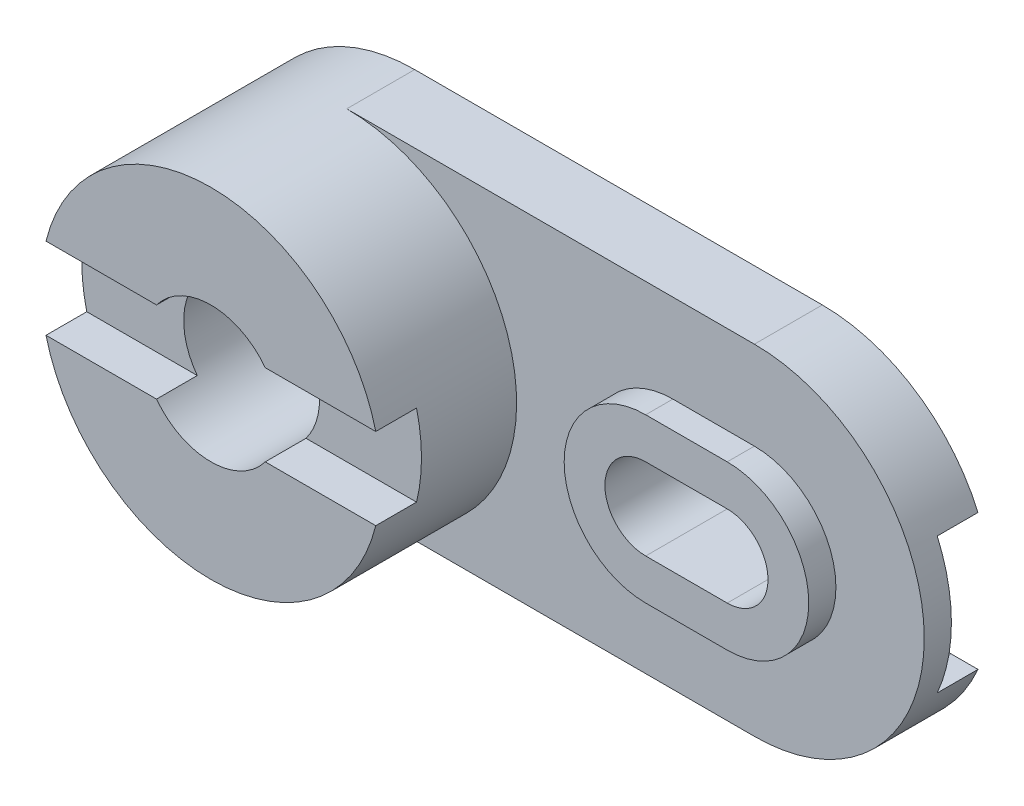
ISO-10303-21;
HEADER;
FILE_DESCRIPTION(('STEP AP214'),'2;1');
FILE_NAME('part.step','',(''),(''),'','','');
FILE_SCHEMA(('AUTOMOTIVE_DESIGN { 1 0 10303 214 1 1 1 1 }'));
ENDSEC;
DATA;
#1=APPLICATION_CONTEXT('core data for automotive mechanical design processes');
#2=APPLICATION_PROTOCOL_DEFINITION('international standard','automotive_design',2000,#1);
#3=PRODUCT_CONTEXT('',#1,'mechanical');
#4=PRODUCT('Part','Part','',(#3));
#5=PRODUCT_RELATED_PRODUCT_CATEGORY('part','',(#4));
#6=PRODUCT_DEFINITION_FORMATION('','',#4);
#7=PRODUCT_DEFINITION_CONTEXT('part definition',#1,'design');
#8=PRODUCT_DEFINITION('design','',#6,#7);
#9=PRODUCT_DEFINITION_SHAPE('','',#8);
#10=(LENGTH_UNIT() NAMED_UNIT(*) SI_UNIT(.MILLI.,.METRE.));
#11=(NAMED_UNIT(*) PLANE_ANGLE_UNIT() SI_UNIT($,.RADIAN.));
#12=(NAMED_UNIT(*) SI_UNIT($,.STERADIAN.) SOLID_ANGLE_UNIT());
#13=UNCERTAINTY_MEASURE_WITH_UNIT(LENGTH_MEASURE(1.E-05),#10,'distance_accuracy_value','');
#14=(GEOMETRIC_REPRESENTATION_CONTEXT(3) GLOBAL_UNCERTAINTY_ASSIGNED_CONTEXT((#13)) GLOBAL_UNIT_ASSIGNED_CONTEXT((#10,
#11,#12)) REPRESENTATION_CONTEXT('',''));
#15=CARTESIAN_POINT('',(0.,0.,0.));
#16=DIRECTION('',(0.,0.,1.));
#17=DIRECTION('',(1.,0.,0.));
#18=AXIS2_PLACEMENT_3D('',#15,#16,#17);
#19=CARTESIAN_POINT('',(60.,0.,10.));
#20=DIRECTION('',(0.,0.,-1.));
#21=DIRECTION('',(-1.,0.,0.));
#22=AXIS2_PLACEMENT_3D('',#19,#20,#21);
#23=CYLINDRICAL_SURFACE('',#22,25.);
#24=DIRECTION('',(0.,0.,1.));
#25=VECTOR('',#24,1.);
#26=CARTESIAN_POINT('',(82.9128784747792,-9.99999999999999,-168.123744974859));
#27=LINE('',#26,#25);
#28=CARTESIAN_POINT('',(82.9128784747792,-9.99999999999999,0.));
#29=VERTEX_POINT('',#28);
#30=CARTESIAN_POINT('',(82.9128784747792,-9.99999999999999,6.));
#31=VERTEX_POINT('',#30);
#32=EDGE_CURVE('E61',#29,#31,#27,.T.);
#33=ORIENTED_EDGE('',*,*,#32,.T.);
#34=CARTESIAN_POINT('',(60.,0.,6.));
#35=DIRECTION('',(0.,0.,1.));
#36=DIRECTION('',(1.,0.,0.));
#37=AXIS2_PLACEMENT_3D('',#34,#35,#36);
#38=CIRCLE('',#37,25.);
#39=CARTESIAN_POINT('',(82.9128784747792,10.,6.));
#40=VERTEX_POINT('',#39);
#41=EDGE_CURVE('E56',#31,#40,#38,.T.);
#42=ORIENTED_EDGE('',*,*,#41,.T.);
#43=DIRECTION('',(0.,0.,1.));
#44=VECTOR('',#43,1.);
#45=CARTESIAN_POINT('',(82.9128784747792,10.,-168.123744974859));
#46=LINE('',#45,#44);
#47=CARTESIAN_POINT('',(82.9128784747792,10.,0.));
#48=VERTEX_POINT('',#47);
#49=EDGE_CURVE('E230',#48,#40,#46,.T.);
#50=ORIENTED_EDGE('',*,*,#49,.F.);
#51=CARTESIAN_POINT('',(60.,0.,0.));
#52=DIRECTION('',(0.,0.,1.));
#53=DIRECTION('',(1.,0.,0.));
#54=AXIS2_PLACEMENT_3D('',#51,#52,#53);
#55=CIRCLE('',#54,25.);
#56=CARTESIAN_POINT('',(60.,25.,0.));
#57=VERTEX_POINT('',#56);
#58=EDGE_CURVE('E213',#48,#57,#55,.T.);
#59=ORIENTED_EDGE('',*,*,#58,.T.);
#60=DIRECTION('',(0.,0.,-1.));
#61=VECTOR('',#60,1.);
#62=CARTESIAN_POINT('',(60.,25.,10.));
#63=LINE('',#62,#61);
#64=CARTESIAN_POINT('',(60.,25.,10.));
#65=VERTEX_POINT('',#64);
#66=EDGE_CURVE('E385',#65,#57,#63,.T.);
#67=ORIENTED_EDGE('',*,*,#66,.F.);
#68=CARTESIAN_POINT('',(60.,0.,10.));
#69=DIRECTION('',(0.,0.,1.));
#70=DIRECTION('',(1.,0.,0.));
#71=AXIS2_PLACEMENT_3D('',#68,#69,#70);
#72=CIRCLE('',#71,25.);
#73=CARTESIAN_POINT('',(60.,-25.,10.));
#74=VERTEX_POINT('',#73);
#75=EDGE_CURVE('E381',#74,#65,#72,.T.);
#76=ORIENTED_EDGE('',*,*,#75,.F.);
#77=DIRECTION('',(0.,0.,-1.));
#78=VECTOR('',#77,1.);
#79=CARTESIAN_POINT('',(60.,-25.,10.));
#80=LINE('',#79,#78);
#81=CARTESIAN_POINT('',(60.,-25.,0.));
#82=VERTEX_POINT('',#81);
#83=EDGE_CURVE('E395',#74,#82,#80,.T.);
#84=ORIENTED_EDGE('',*,*,#83,.T.);
#85=EDGE_CURVE('E223',#82,#29,#55,.T.);
#86=ORIENTED_EDGE('',*,*,#85,.T.);
#87=EDGE_LOOP('',(#33,#42,#50,#59,#67,#76,#84,#86));
#88=FACE_BOUND('',#87,.T.);
#89=ADVANCED_FACE('F44',(#88),#23,.T.);
#90=CARTESIAN_POINT('',(60.,0.,0.));
#91=DIRECTION('',(0.,0.,1.));
#92=DIRECTION('',(1.,0.,0.));
#93=AXIS2_PLACEMENT_3D('',#90,#91,#92);
#94=PLANE('',#93);
#95=CARTESIAN_POINT('',(0.,0.,0.));
#96=DIRECTION('',(0.,0.,1.));
#97=DIRECTION('',(1.,0.,0.));
#98=AXIS2_PLACEMENT_3D('',#95,#96,#97);
#99=CIRCLE('',#98,10.);
#100=CARTESIAN_POINT('',(10.,0.,0.));
#101=VERTEX_POINT('',#100);
#102=EDGE_CURVE('E322',#101,#101,#99,.T.);
#103=ORIENTED_EDGE('',*,*,#102,.T.);
#104=EDGE_LOOP('',(#103));
#105=FACE_BOUND('',#104,.T.);
#106=DIRECTION('',(-1.,0.,0.));
#107=VECTOR('',#106,1.);
#108=CARTESIAN_POINT('',(60.,6.,0.));
#109=LINE('',#108,#107);
#110=CARTESIAN_POINT('',(60.,6.,0.));
#111=VERTEX_POINT('',#110);
#112=CARTESIAN_POINT('',(48.,6.,0.));
#113=VERTEX_POINT('',#112);
#114=EDGE_CURVE('E287',#111,#113,#109,.T.);
#115=ORIENTED_EDGE('',*,*,#114,.T.);
#116=CARTESIAN_POINT('',(48.,0.,0.));
#117=DIRECTION('',(0.,0.,1.));
#118=DIRECTION('',(1.,0.,0.));
#119=AXIS2_PLACEMENT_3D('',#116,#117,#118);
#120=CIRCLE('',#119,6.);
#121=CARTESIAN_POINT('',(48.,-6.,0.));
#122=VERTEX_POINT('',#121);
#123=EDGE_CURVE('E286',#113,#122,#120,.T.);
#124=ORIENTED_EDGE('',*,*,#123,.T.);
#125=DIRECTION('',(1.,0.,0.));
#126=VECTOR('',#125,1.);
#127=CARTESIAN_POINT('',(60.,-6.,0.));
#128=LINE('',#127,#126);
#129=CARTESIAN_POINT('',(60.,-6.,0.));
#130=VERTEX_POINT('',#129);
#131=EDGE_CURVE('E274',#122,#130,#128,.T.);
#132=ORIENTED_EDGE('',*,*,#131,.T.);
#133=CARTESIAN_POINT('',(60.,0.,0.));
#134=DIRECTION('',(0.,0.,1.));
#135=DIRECTION('',(1.,0.,0.));
#136=AXIS2_PLACEMENT_3D('',#133,#134,#135);
#137=CIRCLE('',#136,6.);
#138=EDGE_CURVE('E281',#130,#111,#137,.T.);
#139=ORIENTED_EDGE('',*,*,#138,.T.);
#140=EDGE_LOOP('',(#115,#124,#132,#139));
#141=FACE_BOUND('',#140,.T.);
#142=DIRECTION('',(1.,0.,0.));
#143=VECTOR('',#142,1.);
#144=CARTESIAN_POINT('',(82.9128784747792,-9.99999999999999,0.));
#145=LINE('',#144,#143);
#146=CARTESIAN_POINT('',(79.,-9.99999999999999,0.));
#147=VERTEX_POINT('',#146);
#148=EDGE_CURVE('E258',#147,#29,#145,.T.);
#149=ORIENTED_EDGE('',*,*,#148,.T.);
#150=ORIENTED_EDGE('',*,*,#85,.F.);
#151=DIRECTION('',(1.,0.,0.));
#152=VECTOR('',#151,1.);
#153=CARTESIAN_POINT('',(0.,-25.,0.));
#154=LINE('',#153,#152);
#155=CARTESIAN_POINT('',(0.,-25.,0.));
#156=VERTEX_POINT('',#155);
#157=EDGE_CURVE('E389',#156,#82,#154,.T.);
#158=ORIENTED_EDGE('',*,*,#157,.F.);
#159=CARTESIAN_POINT('',(0.,0.,0.));
#160=DIRECTION('',(0.,0.,1.));
#161=DIRECTION('',(1.,0.,0.));
#162=AXIS2_PLACEMENT_3D('',#159,#160,#161);
#163=CIRCLE('',#162,25.);
#164=CARTESIAN_POINT('',(0.,25.,0.));
#165=VERTEX_POINT('',#164);
#166=EDGE_CURVE('E228',#165,#156,#163,.T.);
#167=ORIENTED_EDGE('',*,*,#166,.F.);
#168=DIRECTION('',(-1.,0.,0.));
#169=VECTOR('',#168,1.);
#170=CARTESIAN_POINT('',(60.,25.,0.));
#171=LINE('',#170,#169);
#172=EDGE_CURVE('E224',#57,#165,#171,.T.);
#173=ORIENTED_EDGE('',*,*,#172,.F.);
#174=ORIENTED_EDGE('',*,*,#58,.F.);
#175=DIRECTION('',(-1.,0.,0.));
#176=VECTOR('',#175,1.);
#177=CARTESIAN_POINT('',(79.,10.,0.));
#178=LINE('',#177,#176);
#179=CARTESIAN_POINT('',(79.,10.,0.));
#180=VERTEX_POINT('',#179);
#181=EDGE_CURVE('E216',#48,#180,#178,.T.);
#182=ORIENTED_EDGE('',*,*,#181,.T.);
#183=DIRECTION('',(-1.,0.,0.));
#184=VECTOR('',#183,1.);
#185=CARTESIAN_POINT('',(79.,10.,0.));
#186=LINE('',#185,#184);
#187=CARTESIAN_POINT('',(69.,10.,0.));
#188=VERTEX_POINT('',#187);
#189=EDGE_CURVE('E237',#180,#188,#186,.T.);
#190=ORIENTED_EDGE('',*,*,#189,.T.);
#191=DIRECTION('',(0.,-1.,0.));
#192=VECTOR('',#191,1.);
#193=CARTESIAN_POINT('',(69.,10.,0.));
#194=LINE('',#193,#192);
#195=CARTESIAN_POINT('',(69.,-9.99999999999999,0.));
#196=VERTEX_POINT('',#195);
#197=EDGE_CURVE('E243',#188,#196,#194,.T.);
#198=ORIENTED_EDGE('',*,*,#197,.T.);
#199=DIRECTION('',(1.,0.,0.));
#200=VECTOR('',#199,1.);
#201=CARTESIAN_POINT('',(69.,-9.99999999999999,0.));
#202=LINE('',#201,#200);
#203=EDGE_CURVE('E435',#196,#147,#202,.T.);
#204=ORIENTED_EDGE('',*,*,#203,.T.);
#205=EDGE_LOOP('',(#149,#150,#158,#167,#173,#174,#182,#190,#198,#204));
#206=FACE_BOUND('',#205,.T.);
#207=ADVANCED_FACE('F218',(#105,#141,#206),#94,.F.);
#208=CARTESIAN_POINT('',(60.,0.,10.));
#209=DIRECTION('',(0.,0.,1.));
#210=DIRECTION('',(1.,0.,0.));
#211=AXIS2_PLACEMENT_3D('',#208,#209,#210);
#212=PLANE('',#211);
#213=CARTESIAN_POINT('',(0.,0.,10.));
#214=DIRECTION('',(0.,0.,1.));
#215=DIRECTION('',(1.,0.,0.));
#216=AXIS2_PLACEMENT_3D('',#213,#214,#215);
#217=CIRCLE('',#216,25.);
#218=CARTESIAN_POINT('',(0.,-25.,10.));
#219=VERTEX_POINT('',#218);
#220=CARTESIAN_POINT('',(0.,25.,10.));
#221=VERTEX_POINT('',#220);
#222=EDGE_CURVE('E378',#219,#221,#217,.T.);
#223=ORIENTED_EDGE('',*,*,#222,.F.);
#224=DIRECTION('',(1.,0.,0.));
#225=VECTOR('',#224,1.);
#226=CARTESIAN_POINT('',(0.,-25.,10.));
#227=LINE('',#226,#225);
#228=EDGE_CURVE('E393',#219,#74,#227,.T.);
#229=ORIENTED_EDGE('',*,*,#228,.T.);
#230=ORIENTED_EDGE('',*,*,#75,.T.);
#231=DIRECTION('',(-1.,0.,0.));
#232=VECTOR('',#231,1.);
#233=CARTESIAN_POINT('',(60.,25.,10.));
#234=LINE('',#233,#232);
#235=EDGE_CURVE('E390',#65,#221,#234,.T.);
#236=ORIENTED_EDGE('',*,*,#235,.T.);
#237=EDGE_LOOP('',(#223,#229,#230,#236));
#238=FACE_BOUND('',#237,.T.);
#239=DIRECTION('',(1.,0.,0.));
#240=VECTOR('',#239,1.);
#241=CARTESIAN_POINT('',(48.,-12.,10.));
#242=LINE('',#241,#240);
#243=CARTESIAN_POINT('',(48.,-12.,10.));
#244=VERTEX_POINT('',#243);
#245=CARTESIAN_POINT('',(60.,-12.,10.));
#246=VERTEX_POINT('',#245);
#247=EDGE_CURVE('E306',#244,#246,#242,.T.);
#248=ORIENTED_EDGE('',*,*,#247,.F.);
#249=CARTESIAN_POINT('',(48.,0.,10.));
#250=DIRECTION('',(0.,0.,1.));
#251=DIRECTION('',(1.,0.,0.));
#252=AXIS2_PLACEMENT_3D('',#249,#250,#251);
#253=CIRCLE('',#252,12.);
#254=CARTESIAN_POINT('',(48.,12.,10.));
#255=VERTEX_POINT('',#254);
#256=EDGE_CURVE('E292',#255,#244,#253,.T.);
#257=ORIENTED_EDGE('',*,*,#256,.F.);
#258=DIRECTION('',(-1.,0.,0.));
#259=VECTOR('',#258,1.);
#260=CARTESIAN_POINT('',(48.,12.,10.));
#261=LINE('',#260,#259);
#262=CARTESIAN_POINT('',(60.,12.,10.));
#263=VERTEX_POINT('',#262);
#264=EDGE_CURVE('E300',#263,#255,#261,.T.);
#265=ORIENTED_EDGE('',*,*,#264,.F.);
#266=CARTESIAN_POINT('',(60.,0.,10.));
#267=DIRECTION('',(0.,0.,1.));
#268=DIRECTION('',(1.,0.,0.));
#269=AXIS2_PLACEMENT_3D('',#266,#267,#268);
#270=CIRCLE('',#269,12.);
#271=EDGE_CURVE('E308',#246,#263,#270,.T.);
#272=ORIENTED_EDGE('',*,*,#271,.F.);
#273=EDGE_LOOP('',(#248,#257,#265,#272));
#274=FACE_BOUND('',#273,.T.);
#275=ADVANCED_FACE('F409',(#238,#274),#212,.T.);
#276=CARTESIAN_POINT('',(0.,0.,24.));
#277=DIRECTION('',(0.,0.,1.));
#278=DIRECTION('',(1.,0.,0.));
#279=AXIS2_PLACEMENT_3D('',#276,#277,#278);
#280=PLANE('',#279);
#281=CARTESIAN_POINT('',(0.,0.,24.));
#282=DIRECTION('',(0.,0.,1.));
#283=DIRECTION('',(1.,0.,0.));
#284=AXIS2_PLACEMENT_3D('',#281,#282,#283);
#285=CIRCLE('',#284,10.);
#286=CARTESIAN_POINT('',(-8.,6.,24.));
#287=VERTEX_POINT('',#286);
#288=CARTESIAN_POINT('',(-8.,-6.,24.));
#289=VERTEX_POINT('',#288);
#290=EDGE_CURVE('E11',#287,#289,#285,.T.);
#291=ORIENTED_EDGE('',*,*,#290,.F.);
#292=DIRECTION('',(1.,0.,0.));
#293=VECTOR('',#292,1.);
#294=CARTESIAN_POINT('',(0.,6.,24.));
#295=LINE('',#294,#293);
#296=CARTESIAN_POINT('',(-24.2693221990232,6.,24.));
#297=VERTEX_POINT('',#296);
#298=EDGE_CURVE('E330',#297,#287,#295,.T.);
#299=ORIENTED_EDGE('',*,*,#298,.F.);
#300=CARTESIAN_POINT('',(0.,0.,24.));
#301=DIRECTION('',(0.,0.,1.));
#302=DIRECTION('',(1.,0.,0.));
#303=AXIS2_PLACEMENT_3D('',#300,#301,#302);
#304=CIRCLE('',#303,25.);
#305=CARTESIAN_POINT('',(-24.2693221990232,-6.,24.));
#306=VERTEX_POINT('',#305);
#307=EDGE_CURVE('E332',#297,#306,#304,.T.);
#308=ORIENTED_EDGE('',*,*,#307,.T.);
#309=DIRECTION('',(-1.,0.,0.));
#310=VECTOR('',#309,1.);
#311=CARTESIAN_POINT('',(0.,-6.,24.));
#312=LINE('',#311,#310);
#313=EDGE_CURVE('E331',#289,#306,#312,.T.);
#314=ORIENTED_EDGE('',*,*,#313,.F.);
#315=EDGE_LOOP('',(#291,#299,#308,#314));
#316=FACE_BOUND('',#315,.T.);
#317=ADVANCED_FACE('F465',(#316),#280,.T.);
#318=CARTESIAN_POINT('',(0.,0.,0.));
#319=DIRECTION('',(0.,0.,1.));
#320=DIRECTION('',(1.,0.,0.));
#321=AXIS2_PLACEMENT_3D('',#318,#319,#320);
#322=CYLINDRICAL_SURFACE('',#321,25.);
#323=DIRECTION('',(0.,0.,-1.));
#324=VECTOR('',#323,1.);
#325=CARTESIAN_POINT('',(0.,25.,10.));
#326=LINE('',#325,#324);
#327=EDGE_CURVE('E402',#221,#165,#326,.T.);
#328=ORIENTED_EDGE('',*,*,#327,.T.);
#329=ORIENTED_EDGE('',*,*,#166,.T.);
#330=DIRECTION('',(0.,0.,-1.));
#331=VECTOR('',#330,1.);
#332=CARTESIAN_POINT('',(0.,-25.,10.));
#333=LINE('',#332,#331);
#334=EDGE_CURVE('E400',#219,#156,#333,.T.);
#335=ORIENTED_EDGE('',*,*,#334,.F.);
#336=ORIENTED_EDGE('',*,*,#222,.T.);
#337=EDGE_LOOP('',(#328,#329,#335,#336));
#338=FACE_BOUND('',#337,.T.);
#339=CARTESIAN_POINT('',(0.,0.,30.));
#340=DIRECTION('',(0.,0.,1.));
#341=DIRECTION('',(1.,0.,0.));
#342=AXIS2_PLACEMENT_3D('',#339,#340,#341);
#343=CIRCLE('',#342,25.);
#344=CARTESIAN_POINT('',(-24.2693221990232,-6.,30.));
#345=VERTEX_POINT('',#344);
#346=CARTESIAN_POINT('',(24.2693221990232,-6.,30.));
#347=VERTEX_POINT('',#346);
#348=EDGE_CURVE('E356',#345,#347,#343,.T.);
#349=ORIENTED_EDGE('',*,*,#348,.F.);
#350=DIRECTION('',(0.,0.,1.));
#351=VECTOR('',#350,1.);
#352=CARTESIAN_POINT('',(-24.2693221990232,-6.,24.));
#353=LINE('',#352,#351);
#354=EDGE_CURVE('E366',#306,#345,#353,.T.);
#355=ORIENTED_EDGE('',*,*,#354,.F.);
#356=ORIENTED_EDGE('',*,*,#307,.F.);
#357=DIRECTION('',(0.,0.,1.));
#358=VECTOR('',#357,1.);
#359=CARTESIAN_POINT('',(-24.2693221990232,6.,24.));
#360=LINE('',#359,#358);
#361=CARTESIAN_POINT('',(-24.2693221990232,6.,30.));
#362=VERTEX_POINT('',#361);
#363=EDGE_CURVE('E368',#297,#362,#360,.T.);
#364=ORIENTED_EDGE('',*,*,#363,.T.);
#365=CARTESIAN_POINT('',(24.2693221990232,6.,30.));
#366=VERTEX_POINT('',#365);
#367=EDGE_CURVE('E376',#366,#362,#343,.T.);
#368=ORIENTED_EDGE('',*,*,#367,.F.);
#369=DIRECTION('',(0.,0.,1.));
#370=VECTOR('',#369,1.);
#371=CARTESIAN_POINT('',(24.2693221990232,6.,24.));
#372=LINE('',#371,#370);
#373=CARTESIAN_POINT('',(24.2693221990232,6.,24.));
#374=VERTEX_POINT('',#373);
#375=EDGE_CURVE('E358',#374,#366,#372,.T.);
#376=ORIENTED_EDGE('',*,*,#375,.F.);
#377=CARTESIAN_POINT('',(24.2693221990232,-6.,24.));
#378=VERTEX_POINT('',#377);
#379=EDGE_CURVE('E333',#378,#374,#304,.T.);
#380=ORIENTED_EDGE('',*,*,#379,.F.);
#381=DIRECTION('',(0.,0.,1.));
#382=VECTOR('',#381,1.);
#383=CARTESIAN_POINT('',(24.2693221990232,-6.,24.));
#384=LINE('',#383,#382);
#385=EDGE_CURVE('E360',#378,#347,#384,.T.);
#386=ORIENTED_EDGE('',*,*,#385,.T.);
#387=EDGE_LOOP('',(#349,#355,#356,#364,#368,#376,#380,#386));
#388=FACE_BOUND('',#387,.T.);
#389=ADVANCED_FACE('F484',(#338,#388),#322,.T.);
#390=CARTESIAN_POINT('',(0.,0.,30.));
#391=DIRECTION('',(0.,0.,1.));
#392=DIRECTION('',(1.,0.,0.));
#393=AXIS2_PLACEMENT_3D('',#390,#391,#392);
#394=PLANE('',#393);
#395=ORIENTED_EDGE('',*,*,#348,.T.);
#396=DIRECTION('',(-1.,0.,0.));
#397=VECTOR('',#396,1.);
#398=CARTESIAN_POINT('',(0.,-6.,30.));
#399=LINE('',#398,#397);
#400=CARTESIAN_POINT('',(8.,-6.,30.));
#401=VERTEX_POINT('',#400);
#402=EDGE_CURVE('E326',#347,#401,#399,.T.);
#403=ORIENTED_EDGE('',*,*,#402,.T.);
#404=CARTESIAN_POINT('',(0.,0.,30.));
#405=DIRECTION('',(0.,0.,1.));
#406=DIRECTION('',(1.,0.,0.));
#407=AXIS2_PLACEMENT_3D('',#404,#405,#406);
#408=CIRCLE('',#407,10.);
#409=CARTESIAN_POINT('',(-8.,-6.,30.));
#410=VERTEX_POINT('',#409);
#411=EDGE_CURVE('E352',#410,#401,#408,.T.);
#412=ORIENTED_EDGE('',*,*,#411,.F.);
#413=DIRECTION('',(-1.,0.,0.));
#414=VECTOR('',#413,1.);
#415=CARTESIAN_POINT('',(0.,-6.,30.));
#416=LINE('',#415,#414);
#417=EDGE_CURVE('E346',#410,#345,#416,.T.);
#418=ORIENTED_EDGE('',*,*,#417,.T.);
#419=EDGE_LOOP('',(#395,#403,#412,#418));
#420=FACE_BOUND('',#419,.T.);
#421=ADVANCED_FACE('F473',(#420),#394,.T.);
#422=CARTESIAN_POINT('',(0.,0.,30.));
#423=DIRECTION('',(0.,0.,1.));
#424=DIRECTION('',(1.,0.,0.));
#425=AXIS2_PLACEMENT_3D('',#422,#423,#424);
#426=CIRCLE('',#425,10.);
#427=CARTESIAN_POINT('',(8.,6.,30.));
#428=VERTEX_POINT('',#427);
#429=CARTESIAN_POINT('',(-8.,6.,30.));
#430=VERTEX_POINT('',#429);
#431=EDGE_CURVE('E345',#428,#430,#426,.T.);
#432=ORIENTED_EDGE('',*,*,#431,.F.);
#433=DIRECTION('',(1.,0.,0.));
#434=VECTOR('',#433,1.);
#435=CARTESIAN_POINT('',(0.,6.,30.));
#436=LINE('',#435,#434);
#437=EDGE_CURVE('E321',#428,#366,#436,.T.);
#438=ORIENTED_EDGE('',*,*,#437,.T.);
#439=ORIENTED_EDGE('',*,*,#367,.T.);
#440=DIRECTION('',(1.,0.,0.));
#441=VECTOR('',#440,1.);
#442=CARTESIAN_POINT('',(0.,6.,30.));
#443=LINE('',#442,#441);
#444=EDGE_CURVE('E343',#362,#430,#443,.T.);
#445=ORIENTED_EDGE('',*,*,#444,.T.);
#446=EDGE_LOOP('',(#432,#438,#439,#445));
#447=FACE_BOUND('',#446,.T.);
#448=ADVANCED_FACE('F472',(#447),#394,.T.);
#449=CARTESIAN_POINT('',(60.,25.,10.));
#450=DIRECTION('',(0.,-1.,0.));
#451=DIRECTION('',(0.,0.,-1.));
#452=AXIS2_PLACEMENT_3D('',#449,#450,#451);
#453=PLANE('',#452);
#454=ORIENTED_EDGE('',*,*,#172,.T.);
#455=ORIENTED_EDGE('',*,*,#327,.F.);
#456=ORIENTED_EDGE('',*,*,#235,.F.);
#457=ORIENTED_EDGE('',*,*,#66,.T.);
#458=EDGE_LOOP('',(#454,#455,#456,#457));
#459=FACE_BOUND('',#458,.T.);
#460=ADVANCED_FACE('F401',(#459),#453,.F.);
#461=CARTESIAN_POINT('',(0.,-25.,10.));
#462=DIRECTION('',(0.,1.,0.));
#463=DIRECTION('',(0.,0.,1.));
#464=AXIS2_PLACEMENT_3D('',#461,#462,#463);
#465=PLANE('',#464);
#466=ORIENTED_EDGE('',*,*,#157,.T.);
#467=ORIENTED_EDGE('',*,*,#83,.F.);
#468=ORIENTED_EDGE('',*,*,#228,.F.);
#469=ORIENTED_EDGE('',*,*,#334,.T.);
#470=EDGE_LOOP('',(#466,#467,#468,#469));
#471=FACE_BOUND('',#470,.T.);
#472=ADVANCED_FACE('F411',(#471),#465,.F.);
#473=CARTESIAN_POINT('',(0.,6.,24.));
#474=DIRECTION('',(0.,-1.,0.));
#475=DIRECTION('',(1.,0.,0.));
#476=AXIS2_PLACEMENT_3D('',#473,#474,#475);
#477=PLANE('',#476);
#478=ORIENTED_EDGE('',*,*,#437,.F.);
#479=DIRECTION('',(0.,0.,1.));
#480=VECTOR('',#479,1.);
#481=CARTESIAN_POINT('',(8.,6.,24.));
#482=LINE('',#481,#480);
#483=CARTESIAN_POINT('',(8.,6.,24.));
#484=VERTEX_POINT('',#483);
#485=EDGE_CURVE('E373',#484,#428,#482,.T.);
#486=ORIENTED_EDGE('',*,*,#485,.F.);
#487=DIRECTION('',(1.,0.,0.));
#488=VECTOR('',#487,1.);
#489=CARTESIAN_POINT('',(0.,6.,24.));
#490=LINE('',#489,#488);
#491=EDGE_CURVE('E323',#484,#374,#490,.T.);
#492=ORIENTED_EDGE('',*,*,#491,.T.);
#493=ORIENTED_EDGE('',*,*,#375,.T.);
#494=EDGE_LOOP('',(#478,#486,#492,#493));
#495=FACE_BOUND('',#494,.T.);
#496=ADVANCED_FACE('F469',(#495),#477,.T.);
#497=CARTESIAN_POINT('',(0.,-6.,24.));
#498=DIRECTION('',(0.,1.,0.));
#499=DIRECTION('',(-1.,0.,0.));
#500=AXIS2_PLACEMENT_3D('',#497,#498,#499);
#501=PLANE('',#500);
#502=ORIENTED_EDGE('',*,*,#402,.F.);
#503=ORIENTED_EDGE('',*,*,#385,.F.);
#504=DIRECTION('',(-1.,0.,0.));
#505=VECTOR('',#504,1.);
#506=CARTESIAN_POINT('',(0.,-6.,24.));
#507=LINE('',#506,#505);
#508=CARTESIAN_POINT('',(8.,-6.,24.));
#509=VERTEX_POINT('',#508);
#510=EDGE_CURVE('E340',#378,#509,#507,.T.);
#511=ORIENTED_EDGE('',*,*,#510,.T.);
#512=DIRECTION('',(0.,0.,1.));
#513=VECTOR('',#512,1.);
#514=CARTESIAN_POINT('',(8.,-6.,24.));
#515=LINE('',#514,#513);
#516=EDGE_CURVE('E365',#509,#401,#515,.T.);
#517=ORIENTED_EDGE('',*,*,#516,.T.);
#518=EDGE_LOOP('',(#502,#503,#511,#517));
#519=FACE_BOUND('',#518,.T.);
#520=ADVANCED_FACE('F521',(#519),#501,.T.);
#521=CARTESIAN_POINT('',(0.,0.,24.));
#522=DIRECTION('',(0.,0.,1.));
#523=DIRECTION('',(1.,0.,0.));
#524=AXIS2_PLACEMENT_3D('',#521,#522,#523);
#525=CYLINDRICAL_SURFACE('',#524,10.);
#526=ORIENTED_EDGE('',*,*,#411,.T.);
#527=ORIENTED_EDGE('',*,*,#516,.F.);
#528=EDGE_CURVE('E48',#509,#484,#285,.T.);
#529=ORIENTED_EDGE('',*,*,#528,.T.);
#530=ORIENTED_EDGE('',*,*,#485,.T.);
#531=ORIENTED_EDGE('',*,*,#431,.T.);
#532=DIRECTION('',(0.,0.,1.));
#533=VECTOR('',#532,1.);
#534=CARTESIAN_POINT('',(-8.,6.,24.));
#535=LINE('',#534,#533);
#536=EDGE_CURVE('E371',#287,#430,#535,.T.);
#537=ORIENTED_EDGE('',*,*,#536,.F.);
#538=ORIENTED_EDGE('',*,*,#290,.T.);
#539=DIRECTION('',(0.,0.,1.));
#540=VECTOR('',#539,1.);
#541=CARTESIAN_POINT('',(-8.,-6.,24.));
#542=LINE('',#541,#540);
#543=EDGE_CURVE('E364',#289,#410,#542,.T.);
#544=ORIENTED_EDGE('',*,*,#543,.T.);
#545=EDGE_LOOP('',(#526,#527,#529,#530,#531,#537,#538,#544));
#546=FACE_BOUND('',#545,.T.);
#547=ORIENTED_EDGE('',*,*,#102,.F.);
#548=EDGE_LOOP('',(#547));
#549=FACE_BOUND('',#548,.T.);
#550=ADVANCED_FACE('F513',(#546,#549),#525,.F.);
#551=CARTESIAN_POINT('',(0.,-6.,24.));
#552=DIRECTION('',(0.,1.,0.));
#553=DIRECTION('',(-1.,0.,0.));
#554=AXIS2_PLACEMENT_3D('',#551,#552,#553);
#555=PLANE('',#554);
#556=ORIENTED_EDGE('',*,*,#417,.F.);
#557=ORIENTED_EDGE('',*,*,#543,.F.);
#558=ORIENTED_EDGE('',*,*,#313,.T.);
#559=ORIENTED_EDGE('',*,*,#354,.T.);
#560=EDGE_LOOP('',(#556,#557,#558,#559));
#561=FACE_BOUND('',#560,.T.);
#562=ADVANCED_FACE('F504',(#561),#555,.T.);
#563=CARTESIAN_POINT('',(0.,6.,24.));
#564=DIRECTION('',(0.,-1.,0.));
#565=DIRECTION('',(1.,0.,0.));
#566=AXIS2_PLACEMENT_3D('',#563,#564,#565);
#567=PLANE('',#566);
#568=ORIENTED_EDGE('',*,*,#444,.F.);
#569=ORIENTED_EDGE('',*,*,#363,.F.);
#570=ORIENTED_EDGE('',*,*,#298,.T.);
#571=ORIENTED_EDGE('',*,*,#536,.T.);
#572=EDGE_LOOP('',(#568,#569,#570,#571));
#573=FACE_BOUND('',#572,.T.);
#574=ADVANCED_FACE('F522',(#573),#567,.T.);
#575=ORIENTED_EDGE('',*,*,#528,.F.);
#576=ORIENTED_EDGE('',*,*,#510,.F.);
#577=ORIENTED_EDGE('',*,*,#379,.T.);
#578=ORIENTED_EDGE('',*,*,#491,.F.);
#579=EDGE_LOOP('',(#575,#576,#577,#578));
#580=FACE_BOUND('',#579,.T.);
#581=ADVANCED_FACE('F494',(#580),#280,.T.);
#582=CARTESIAN_POINT('',(48.,0.,14.));
#583=DIRECTION('',(0.,0.,-1.));
#584=DIRECTION('',(-1.,0.,0.));
#585=AXIS2_PLACEMENT_3D('',#582,#583,#584);
#586=CYLINDRICAL_SURFACE('',#585,12.);
#587=ORIENTED_EDGE('',*,*,#256,.T.);
#588=DIRECTION('',(0.,0.,-1.));
#589=VECTOR('',#588,1.);
#590=CARTESIAN_POINT('',(48.,-12.,14.));
#591=LINE('',#590,#589);
#592=CARTESIAN_POINT('',(48.,-12.,14.));
#593=VERTEX_POINT('',#592);
#594=EDGE_CURVE('E316',#593,#244,#591,.T.);
#595=ORIENTED_EDGE('',*,*,#594,.F.);
#596=CARTESIAN_POINT('',(48.,0.,14.));
#597=DIRECTION('',(0.,0.,1.));
#598=DIRECTION('',(1.,0.,0.));
#599=AXIS2_PLACEMENT_3D('',#596,#597,#598);
#600=CIRCLE('',#599,12.);
#601=CARTESIAN_POINT('',(48.,12.,14.));
#602=VERTEX_POINT('',#601);
#603=EDGE_CURVE('E291',#602,#593,#600,.T.);
#604=ORIENTED_EDGE('',*,*,#603,.F.);
#605=DIRECTION('',(0.,0.,-1.));
#606=VECTOR('',#605,1.);
#607=CARTESIAN_POINT('',(48.,12.,14.));
#608=LINE('',#607,#606);
#609=EDGE_CURVE('E303',#602,#255,#608,.T.);
#610=ORIENTED_EDGE('',*,*,#609,.T.);
#611=EDGE_LOOP('',(#587,#595,#604,#610));
#612=FACE_BOUND('',#611,.T.);
#613=ADVANCED_FACE('F528',(#612),#586,.T.);
#614=CARTESIAN_POINT('',(48.,-12.,14.));
#615=DIRECTION('',(0.,1.,0.));
#616=DIRECTION('',(0.,0.,1.));
#617=AXIS2_PLACEMENT_3D('',#614,#615,#616);
#618=PLANE('',#617);
#619=ORIENTED_EDGE('',*,*,#247,.T.);
#620=DIRECTION('',(0.,0.,-1.));
#621=VECTOR('',#620,1.);
#622=CARTESIAN_POINT('',(60.,-12.,14.));
#623=LINE('',#622,#621);
#624=CARTESIAN_POINT('',(60.,-12.,14.));
#625=VERTEX_POINT('',#624);
#626=EDGE_CURVE('E317',#625,#246,#623,.T.);
#627=ORIENTED_EDGE('',*,*,#626,.F.);
#628=DIRECTION('',(1.,0.,0.));
#629=VECTOR('',#628,1.);
#630=CARTESIAN_POINT('',(48.,-12.,14.));
#631=LINE('',#630,#629);
#632=EDGE_CURVE('E298',#593,#625,#631,.T.);
#633=ORIENTED_EDGE('',*,*,#632,.F.);
#634=ORIENTED_EDGE('',*,*,#594,.T.);
#635=EDGE_LOOP('',(#619,#627,#633,#634));
#636=FACE_BOUND('',#635,.T.);
#637=ADVANCED_FACE('F536',(#636),#618,.F.);
#638=CARTESIAN_POINT('',(60.,0.,14.));
#639=DIRECTION('',(0.,0.,-1.));
#640=DIRECTION('',(-1.,0.,0.));
#641=AXIS2_PLACEMENT_3D('',#638,#639,#640);
#642=CYLINDRICAL_SURFACE('',#641,12.);
#643=ORIENTED_EDGE('',*,*,#271,.T.);
#644=DIRECTION('',(0.,0.,-1.));
#645=VECTOR('',#644,1.);
#646=CARTESIAN_POINT('',(60.,12.,14.));
#647=LINE('',#646,#645);
#648=CARTESIAN_POINT('',(60.,12.,14.));
#649=VERTEX_POINT('',#648);
#650=EDGE_CURVE('E313',#649,#263,#647,.T.);
#651=ORIENTED_EDGE('',*,*,#650,.F.);
#652=CARTESIAN_POINT('',(60.,0.,14.));
#653=DIRECTION('',(0.,0.,1.));
#654=DIRECTION('',(1.,0.,0.));
#655=AXIS2_PLACEMENT_3D('',#652,#653,#654);
#656=CIRCLE('',#655,12.);
#657=EDGE_CURVE('E299',#625,#649,#656,.T.);
#658=ORIENTED_EDGE('',*,*,#657,.F.);
#659=ORIENTED_EDGE('',*,*,#626,.T.);
#660=EDGE_LOOP('',(#643,#651,#658,#659));
#661=FACE_BOUND('',#660,.T.);
#662=ADVANCED_FACE('F541',(#661),#642,.T.);
#663=CARTESIAN_POINT('',(48.,12.,14.));
#664=DIRECTION('',(0.,-1.,0.));
#665=DIRECTION('',(0.,0.,-1.));
#666=AXIS2_PLACEMENT_3D('',#663,#664,#665);
#667=PLANE('',#666);
#668=ORIENTED_EDGE('',*,*,#264,.T.);
#669=ORIENTED_EDGE('',*,*,#609,.F.);
#670=DIRECTION('',(-1.,0.,0.));
#671=VECTOR('',#670,1.);
#672=CARTESIAN_POINT('',(48.,12.,14.));
#673=LINE('',#672,#671);
#674=EDGE_CURVE('E301',#649,#602,#673,.T.);
#675=ORIENTED_EDGE('',*,*,#674,.F.);
#676=ORIENTED_EDGE('',*,*,#650,.T.);
#677=EDGE_LOOP('',(#668,#669,#675,#676));
#678=FACE_BOUND('',#677,.T.);
#679=ADVANCED_FACE('F549',(#678),#667,.F.);
#680=CARTESIAN_POINT('',(48.,0.,14.));
#681=DIRECTION('',(0.,0.,1.));
#682=DIRECTION('',(1.,0.,0.));
#683=AXIS2_PLACEMENT_3D('',#680,#681,#682);
#684=PLANE('',#683);
#685=CARTESIAN_POINT('',(48.,0.,14.));
#686=DIRECTION('',(0.,0.,1.));
#687=DIRECTION('',(1.,0.,0.));
#688=AXIS2_PLACEMENT_3D('',#685,#686,#687);
#689=CIRCLE('',#688,6.);
#690=CARTESIAN_POINT('',(48.,6.,14.));
#691=VERTEX_POINT('',#690);
#692=CARTESIAN_POINT('',(48.,-6.,14.));
#693=VERTEX_POINT('',#692);
#694=EDGE_CURVE('E259',#691,#693,#689,.T.);
#695=ORIENTED_EDGE('',*,*,#694,.F.);
#696=DIRECTION('',(-1.,0.,0.));
#697=VECTOR('',#696,1.);
#698=CARTESIAN_POINT('',(48.,6.,14.));
#699=LINE('',#698,#697);
#700=CARTESIAN_POINT('',(60.,6.,14.));
#701=VERTEX_POINT('',#700);
#702=EDGE_CURVE('E270',#701,#691,#699,.T.);
#703=ORIENTED_EDGE('',*,*,#702,.F.);
#704=CARTESIAN_POINT('',(60.,0.,14.));
#705=DIRECTION('',(0.,0.,1.));
#706=DIRECTION('',(1.,0.,0.));
#707=AXIS2_PLACEMENT_3D('',#704,#705,#706);
#708=CIRCLE('',#707,6.);
#709=CARTESIAN_POINT('',(60.,-6.,14.));
#710=VERTEX_POINT('',#709);
#711=EDGE_CURVE('E264',#710,#701,#708,.T.);
#712=ORIENTED_EDGE('',*,*,#711,.F.);
#713=DIRECTION('',(1.,0.,0.));
#714=VECTOR('',#713,1.);
#715=CARTESIAN_POINT('',(60.,-6.,14.));
#716=LINE('',#715,#714);
#717=EDGE_CURVE('E265',#693,#710,#716,.T.);
#718=ORIENTED_EDGE('',*,*,#717,.F.);
#719=EDGE_LOOP('',(#695,#703,#712,#718));
#720=FACE_BOUND('',#719,.T.);
#721=ORIENTED_EDGE('',*,*,#603,.T.);
#722=ORIENTED_EDGE('',*,*,#632,.T.);
#723=ORIENTED_EDGE('',*,*,#657,.T.);
#724=ORIENTED_EDGE('',*,*,#674,.T.);
#725=EDGE_LOOP('',(#721,#722,#723,#724));
#726=FACE_BOUND('',#725,.T.);
#727=ADVANCED_FACE('F553',(#720,#726),#684,.T.);
#728=CARTESIAN_POINT('',(48.,0.,-6.));
#729=DIRECTION('',(0.,0.,1.));
#730=DIRECTION('',(1.,0.,0.));
#731=AXIS2_PLACEMENT_3D('',#728,#729,#730);
#732=CYLINDRICAL_SURFACE('',#731,6.);
#733=DIRECTION('',(0.,0.,1.));
#734=VECTOR('',#733,1.);
#735=CARTESIAN_POINT('',(48.,6.,-6.));
#736=LINE('',#735,#734);
#737=EDGE_CURVE('E275',#113,#691,#736,.T.);
#738=ORIENTED_EDGE('',*,*,#737,.T.);
#739=ORIENTED_EDGE('',*,*,#694,.T.);
#740=DIRECTION('',(0.,0.,1.));
#741=VECTOR('',#740,1.);
#742=CARTESIAN_POINT('',(48.,-6.,-6.));
#743=LINE('',#742,#741);
#744=EDGE_CURVE('E272',#122,#693,#743,.T.);
#745=ORIENTED_EDGE('',*,*,#744,.F.);
#746=ORIENTED_EDGE('',*,*,#123,.F.);
#747=EDGE_LOOP('',(#738,#739,#745,#746));
#748=FACE_BOUND('',#747,.T.);
#749=ADVANCED_FACE('F554',(#748),#732,.F.);
#750=CARTESIAN_POINT('',(48.,6.,-6.));
#751=DIRECTION('',(0.,1.,0.));
#752=DIRECTION('',(0.,0.,1.));
#753=AXIS2_PLACEMENT_3D('',#750,#751,#752);
#754=PLANE('',#753);
#755=DIRECTION('',(0.,0.,1.));
#756=VECTOR('',#755,1.);
#757=CARTESIAN_POINT('',(60.,6.,-6.));
#758=LINE('',#757,#756);
#759=EDGE_CURVE('E273',#111,#701,#758,.T.);
#760=ORIENTED_EDGE('',*,*,#759,.T.);
#761=ORIENTED_EDGE('',*,*,#702,.T.);
#762=ORIENTED_EDGE('',*,*,#737,.F.);
#763=ORIENTED_EDGE('',*,*,#114,.F.);
#764=EDGE_LOOP('',(#760,#761,#762,#763));
#765=FACE_BOUND('',#764,.T.);
#766=ADVANCED_FACE('F559',(#765),#754,.F.);
#767=CARTESIAN_POINT('',(60.,0.,-6.));
#768=DIRECTION('',(0.,0.,1.));
#769=DIRECTION('',(1.,0.,0.));
#770=AXIS2_PLACEMENT_3D('',#767,#768,#769);
#771=CYLINDRICAL_SURFACE('',#770,6.);
#772=DIRECTION('',(0.,0.,1.));
#773=VECTOR('',#772,1.);
#774=CARTESIAN_POINT('',(60.,-6.,-6.));
#775=LINE('',#774,#773);
#776=EDGE_CURVE('E280',#130,#710,#775,.T.);
#777=ORIENTED_EDGE('',*,*,#776,.T.);
#778=ORIENTED_EDGE('',*,*,#711,.T.);
#779=ORIENTED_EDGE('',*,*,#759,.F.);
#780=ORIENTED_EDGE('',*,*,#138,.F.);
#781=EDGE_LOOP('',(#777,#778,#779,#780));
#782=FACE_BOUND('',#781,.T.);
#783=ADVANCED_FACE('F563',(#782),#771,.F.);
#784=CARTESIAN_POINT('',(60.,-6.,-6.));
#785=DIRECTION('',(0.,-1.,0.));
#786=DIRECTION('',(0.,0.,-1.));
#787=AXIS2_PLACEMENT_3D('',#784,#785,#786);
#788=PLANE('',#787);
#789=ORIENTED_EDGE('',*,*,#744,.T.);
#790=ORIENTED_EDGE('',*,*,#717,.T.);
#791=ORIENTED_EDGE('',*,*,#776,.F.);
#792=ORIENTED_EDGE('',*,*,#131,.F.);
#793=EDGE_LOOP('',(#789,#790,#791,#792));
#794=FACE_BOUND('',#793,.T.);
#795=ADVANCED_FACE('F561',(#794),#788,.F.);
#796=CARTESIAN_POINT('',(82.9128784747792,-9.99999999999999,-168.123744974859));
#797=DIRECTION('',(0.,1.,0.));
#798=DIRECTION('',(0.,0.,1.));
#799=AXIS2_PLACEMENT_3D('',#796,#797,#798);
#800=PLANE('',#799);
#801=ORIENTED_EDGE('',*,*,#148,.F.);
#802=DIRECTION('',(0.,0.,1.));
#803=VECTOR('',#802,1.);
#804=CARTESIAN_POINT('',(79.,-9.99999999999999,-168.123744974859));
#805=LINE('',#804,#803);
#806=CARTESIAN_POINT('',(79.,-9.99999999999999,6.));
#807=VERTEX_POINT('',#806);
#808=EDGE_CURVE('E251',#147,#807,#805,.T.);
#809=ORIENTED_EDGE('',*,*,#808,.T.);
#810=DIRECTION('',(1.,0.,0.));
#811=VECTOR('',#810,1.);
#812=CARTESIAN_POINT('',(82.9128784747792,-9.99999999999999,6.00000000000001));
#813=LINE('',#812,#811);
#814=EDGE_CURVE('E231',#807,#31,#813,.T.);
#815=ORIENTED_EDGE('',*,*,#814,.T.);
#816=ORIENTED_EDGE('',*,*,#32,.F.);
#817=EDGE_LOOP('',(#801,#809,#815,#816));
#818=FACE_BOUND('',#817,.T.);
#819=ADVANCED_FACE('F420',(#818),#800,.T.);
#820=CARTESIAN_POINT('',(69.,-9.99999999999999,-168.123744974859));
#821=DIRECTION('',(0.,1.,0.));
#822=DIRECTION('',(0.,0.,1.));
#823=AXIS2_PLACEMENT_3D('',#820,#821,#822);
#824=PLANE('',#823);
#825=ORIENTED_EDGE('',*,*,#203,.F.);
#826=DIRECTION('',(0.,0.,1.));
#827=VECTOR('',#826,1.);
#828=CARTESIAN_POINT('',(69.,-9.99999999999999,-168.123744974859));
#829=LINE('',#828,#827);
#830=CARTESIAN_POINT('',(69.,-9.99999999999999,6.));
#831=VERTEX_POINT('',#830);
#832=EDGE_CURVE('E252',#196,#831,#829,.T.);
#833=ORIENTED_EDGE('',*,*,#832,.T.);
#834=DIRECTION('',(1.,0.,0.));
#835=VECTOR('',#834,1.);
#836=CARTESIAN_POINT('',(69.,-9.99999999999999,6.00000000000001));
#837=LINE('',#836,#835);
#838=EDGE_CURVE('E422',#831,#807,#837,.T.);
#839=ORIENTED_EDGE('',*,*,#838,.T.);
#840=ORIENTED_EDGE('',*,*,#808,.F.);
#841=EDGE_LOOP('',(#825,#833,#839,#840));
#842=FACE_BOUND('',#841,.T.);
#843=ADVANCED_FACE('F437',(#842),#824,.T.);
#844=CARTESIAN_POINT('',(69.,10.,-168.123744974859));
#845=DIRECTION('',(1.,0.,0.));
#846=DIRECTION('',(0.,0.,-1.));
#847=AXIS2_PLACEMENT_3D('',#844,#845,#846);
#848=PLANE('',#847);
#849=ORIENTED_EDGE('',*,*,#197,.F.);
#850=DIRECTION('',(0.,0.,1.));
#851=VECTOR('',#850,1.);
#852=CARTESIAN_POINT('',(69.,10.,-168.123744974859));
#853=LINE('',#852,#851);
#854=CARTESIAN_POINT('',(69.,10.,6.));
#855=VERTEX_POINT('',#854);
#856=EDGE_CURVE('E247',#188,#855,#853,.T.);
#857=ORIENTED_EDGE('',*,*,#856,.T.);
#858=DIRECTION('',(0.,-1.,0.));
#859=VECTOR('',#858,1.);
#860=CARTESIAN_POINT('',(69.,10.,6.00000000000001));
#861=LINE('',#860,#859);
#862=EDGE_CURVE('E425',#855,#831,#861,.T.);
#863=ORIENTED_EDGE('',*,*,#862,.T.);
#864=ORIENTED_EDGE('',*,*,#832,.F.);
#865=EDGE_LOOP('',(#849,#857,#863,#864));
#866=FACE_BOUND('',#865,.T.);
#867=ADVANCED_FACE('F439',(#866),#848,.T.);
#868=CARTESIAN_POINT('',(79.,10.,-168.123744974859));
#869=DIRECTION('',(0.,-1.,0.));
#870=DIRECTION('',(0.,0.,-1.));
#871=AXIS2_PLACEMENT_3D('',#868,#869,#870);
#872=PLANE('',#871);
#873=ORIENTED_EDGE('',*,*,#189,.F.);
#874=DIRECTION('',(0.,0.,1.));
#875=VECTOR('',#874,1.);
#876=CARTESIAN_POINT('',(79.,10.,-168.123744974859));
#877=LINE('',#876,#875);
#878=CARTESIAN_POINT('',(79.,10.,6.));
#879=VERTEX_POINT('',#878);
#880=EDGE_CURVE('E235',#180,#879,#877,.T.);
#881=ORIENTED_EDGE('',*,*,#880,.T.);
#882=DIRECTION('',(-1.,0.,0.));
#883=VECTOR('',#882,1.);
#884=CARTESIAN_POINT('',(79.,10.,6.00000000000001));
#885=LINE('',#884,#883);
#886=EDGE_CURVE('E241',#879,#855,#885,.T.);
#887=ORIENTED_EDGE('',*,*,#886,.T.);
#888=ORIENTED_EDGE('',*,*,#856,.F.);
#889=EDGE_LOOP('',(#873,#881,#887,#888));
#890=FACE_BOUND('',#889,.T.);
#891=ADVANCED_FACE('F442',(#890),#872,.T.);
#892=CARTESIAN_POINT('',(79.,10.,-168.123744974859));
#893=DIRECTION('',(0.,-1.,0.));
#894=DIRECTION('',(0.,0.,-1.));
#895=AXIS2_PLACEMENT_3D('',#892,#893,#894);
#896=PLANE('',#895);
#897=ORIENTED_EDGE('',*,*,#181,.F.);
#898=ORIENTED_EDGE('',*,*,#49,.T.);
#899=DIRECTION('',(-1.,0.,0.));
#900=VECTOR('',#899,1.);
#901=CARTESIAN_POINT('',(79.,10.,6.00000000000001));
#902=LINE('',#901,#900);
#903=EDGE_CURVE('E238',#40,#879,#902,.T.);
#904=ORIENTED_EDGE('',*,*,#903,.T.);
#905=ORIENTED_EDGE('',*,*,#880,.F.);
#906=EDGE_LOOP('',(#897,#898,#904,#905));
#907=FACE_BOUND('',#906,.T.);
#908=ADVANCED_FACE('F236',(#907),#896,.T.);
#909=CARTESIAN_POINT('',(60.,0.,6.));
#910=DIRECTION('',(0.,0.,1.));
#911=DIRECTION('',(1.,0.,0.));
#912=AXIS2_PLACEMENT_3D('',#909,#910,#911);
#913=PLANE('',#912);
#914=ORIENTED_EDGE('',*,*,#903,.F.);
#915=ORIENTED_EDGE('',*,*,#41,.F.);
#916=ORIENTED_EDGE('',*,*,#814,.F.);
#917=ORIENTED_EDGE('',*,*,#838,.F.);
#918=ORIENTED_EDGE('',*,*,#862,.F.);
#919=ORIENTED_EDGE('',*,*,#886,.F.);
#920=EDGE_LOOP('',(#914,#915,#916,#917,#918,#919));
#921=FACE_BOUND('',#920,.T.);
#922=ADVANCED_FACE('F441',(#921),#913,.F.);
#923=CLOSED_SHELL('',(#89,#207,#275,#317,#389,#421,#448,#460,#472,#496,#520,#550,#562,#574,#581,
#613,#637,#662,#679,#727,#749,#766,#783,#795,#819,#843,#867,#891,#908,#922));
#924=MANIFOLD_SOLID_BREP('B2',#923);
#925=ADVANCED_BREP_SHAPE_REPRESENTATION('',(#18,#924),#14);
#926=SHAPE_DEFINITION_REPRESENTATION(#9,#925);
ENDSEC;
END-ISO-10303-21;
